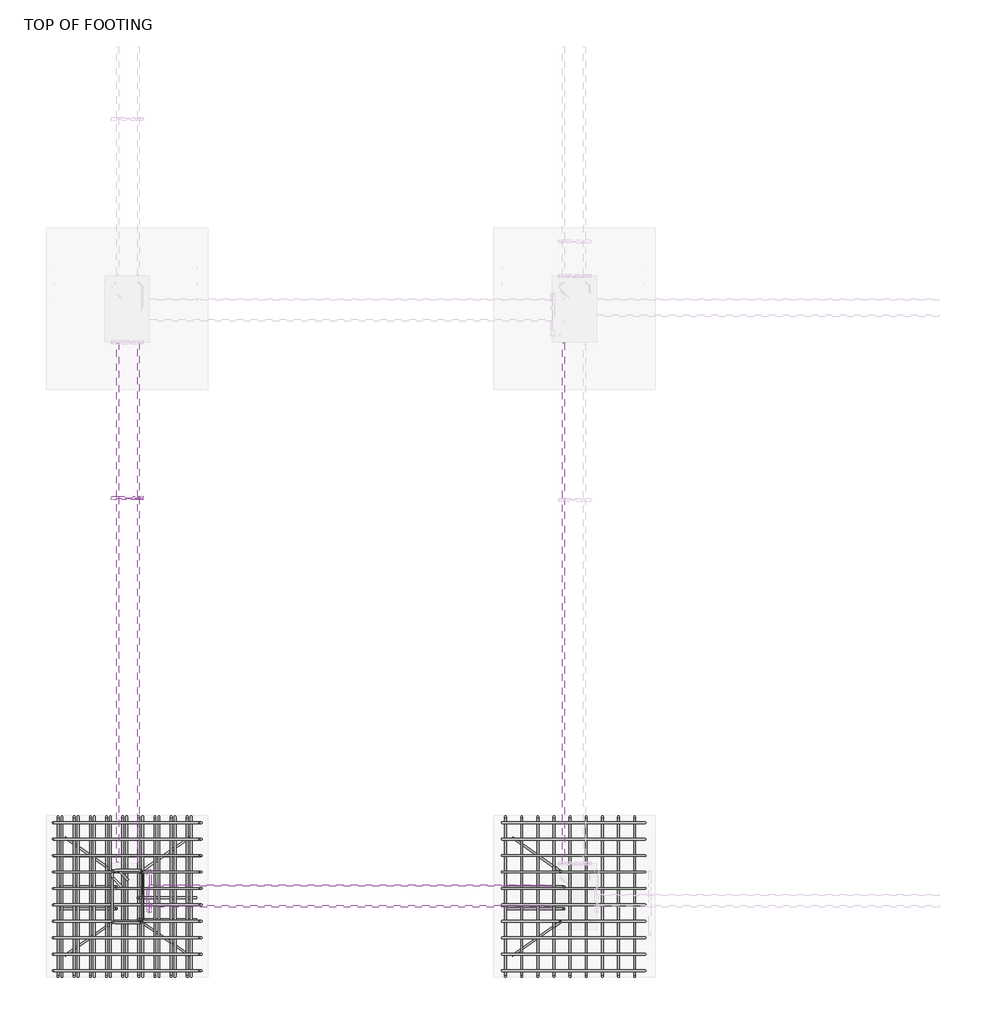
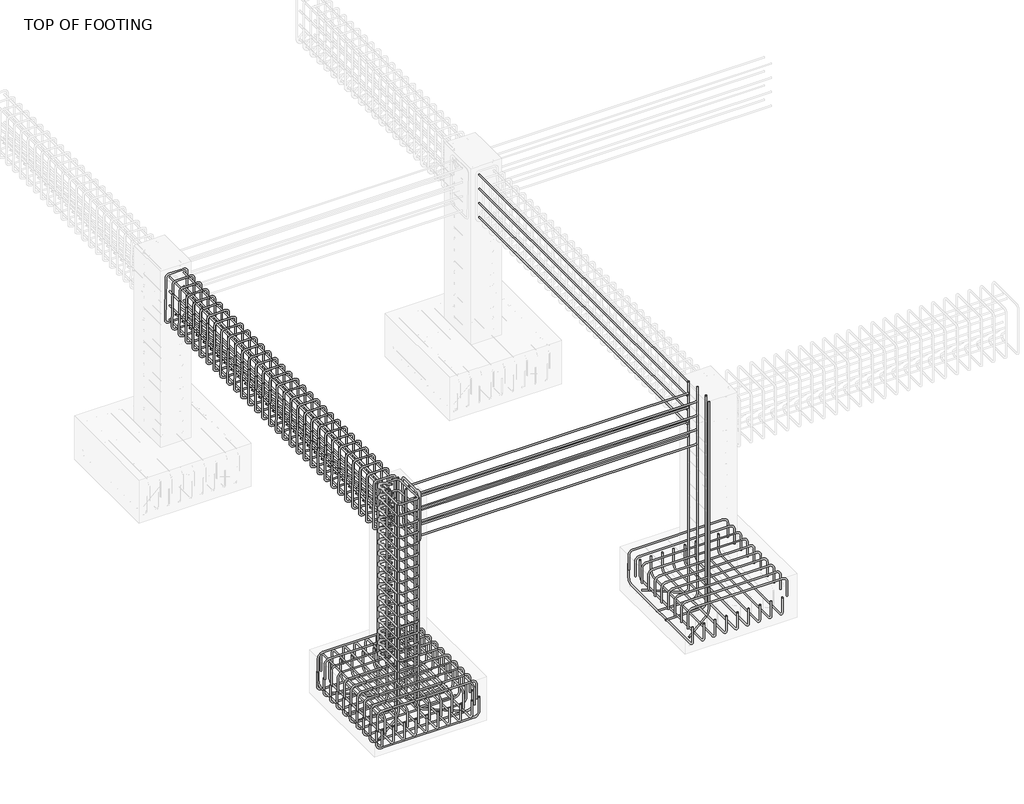
# One storey, part 2 of 18: 23 reinforcing bars.
"""IFC4 building model written with IfcOpenShell, lengths in millimetres."""

from ifc_helpers import new_model, si_unit, point, frame, origin, place, context, project, spatial, polyline, circle_curve, trimmed, segment, composite_curve, source, transform, mapped, element, save
from ifc_brep_helpers import swept_disk

model = new_model("IFC4")

# Units and contexts
model_context = context("Model", 3, world=origin())
ifc_project = project(units=[si_unit("LENGTHUNIT", "METRE", prefix="MILLI")], contexts=[model_context])

# Site, building, storey
site = spatial("IfcSite", under=ifc_project)
building = spatial("IfcBuilding", under=site)
storey = spatial("IfcBuildingStorey", under=building, Name="TOP OF FOOTING", Elevation=-1828.8)

# Reinforcing bars
placement = place(None, origin())
reinforcing_bar_shape = source(origin(), model_context, "Body", "SolidModel", [
    swept_disk(composite_curve([segment(polyline([(-11115.9859643, 5574.8477614, -40.0), (-11115.9859643, 5574.8477614, -2185.2530621)]), True, "CONTINUOUS"), segment(trimmed(circle_curve(frame((-11162.3359643, 5574.8477614, -2185.2530621), z_axis=(0.0, 1.0, 0.0), x_axis=(46.350000000000364, 0.0, 0.0)), 46.35), [point((-11115.9859643, 5574.8477614, -2185.2530621))], [point((-11162.3359643, 5574.8477614, -2231.6030621))], True, "CARTESIAN"), True, "CONTINUOUS"), segment(polyline([(-11162.3359643, 5574.8477614, -2231.6030621), (-11513.5126143, 5574.8477614, -2231.6030621)]), True, "CONTINUOUS")], self_intersect=False), 6.35),
])
element("IfcReinforcingBar", 1, at=placement, inside=storey, context=model_context, shape_type="MappedRepresentation", body=[
    mapped(reinforcing_bar_shape, transform((0.0, 0.0, 0.0), x_axis=(1.0, 0.0, 0.0), y_axis=(0.0, 1.0, 0.0), z_axis=(0.0, 0.0, 1.0))),
    mapped(reinforcing_bar_shape, transform((0.0, 148.3194112, 0.0), x_axis=(1.0, 0.0, 0.0), y_axis=(0.0, 1.0, 0.0), z_axis=(0.0, 0.0, 1.0))),
])
element("IfcReinforcingBar", 2, at=placement, inside=storey, context=model_context, shape_type="SolidModel", body=[
    swept_disk(composite_curve([segment(polyline([(-11140.9859643, 5830.3098681, -40.0), (-11140.9859643, 5830.3098681, -2185.2530621)]), True, "CONTINUOUS"), segment(trimmed(circle_curve(frame((-11178.9536616, 5856.895136, -2185.2530621), z_axis=(0.5735764363510553, 0.8191520442889855, 0.0), x_axis=(37.96769730000051, -26.585267899999963, 0.0)), 46.35), [point((-11140.9859643, 5830.3098681, -2185.2530621))], [point((-11178.9536616, 5856.895136, -2231.6030621))], True, "CARTESIAN"), True, "CONTINUOUS"), segment(polyline([(-11178.9536616, 5856.895136, -2231.6030621), (-11466.6207323, 6058.3217874, -2231.6030621)]), True, "CONTINUOUS")], self_intersect=False), 6.35),
])
reinforcing_bar_2_shape = source(origin(), model_context, "Body", "SolidModel", [
    swept_disk(composite_curve([segment(polyline([(-11036.6954038, 5770.3841028, -1782.45), (-11092.4389667, 5826.1276657, -1782.45)]), True, "CONTINUOUS"), segment(trimmed(circle_curve(frame((-11114.6067643, 5803.9598681, -1782.45), z_axis=(0.0, 0.0, 1.0), x_axis=(22.167797600000995, 22.167797600000085, 0.0)), 31.35), [point((-11092.4389667, 5826.1276657, -1782.45))], [point((-11145.9567643, 5803.9598681, -1782.45))], True, "CARTESIAN"), True, "CONTINUOUS"), segment(polyline([(-11145.9567643, 5803.9598681, -1782.45), (-11145.9567643, 5509.3598681, -1782.45)]), True, "CONTINUOUS"), segment(trimmed(circle_curve(frame((-11114.6067643, 5509.3598681, -1782.45), z_axis=(0.0, 0.0, 1.0), x_axis=(-31.349999999998545, 0.0, 0.0)), 31.35), [point((-11145.9567643, 5509.3598681, -1782.45))], [point((-11114.6067643, 5478.0098681, -1782.45))], True, "CARTESIAN"), True, "CONTINUOUS"), segment(polyline([(-11114.6067643, 5478.0098681, -1782.45), (-10970.0067643, 5478.0098681, -1782.45)]), True, "CONTINUOUS"), segment(trimmed(circle_curve(frame((-10970.0067643, 5509.3400831, -1783.5636125), z_axis=(0.0, 0.03552192833448201, 0.9993688971583016), x_axis=(0.0, -31.330214999999953, 1.1136125000000447)), 31.35), [point((-10970.0067643, 5478.0098681, -1782.45))], [point((-10938.6567643, 5509.3400831, -1783.5636125))], True, "CARTESIAN"), True, "CONTINUOUS"), segment(polyline([(-10938.6567643, 5509.3400831, -1783.5636125), (-10938.6567643, 5803.9796532, -1794.0363875)]), True, "CONTINUOUS"), segment(trimmed(circle_curve(frame((-10970.0067643, 5803.9796532, -1794.0363875), z_axis=(0.0, 0.03552192833448201, 0.9993688971583016), x_axis=(31.350000000000364, 0.0, 0.0)), 31.35), [point((-10938.6567643, 5803.9796532, -1794.0363875))], [point((-10970.0067643, 5835.3098681, -1795.15))], True, "CARTESIAN"), True, "CONTINUOUS"), segment(polyline([(-10970.0067643, 5835.3098681, -1795.15), (-11114.6067643, 5835.3098681, -1795.15)]), True, "CONTINUOUS"), segment(trimmed(circle_curve(frame((-11114.6067643, 5803.9598681, -1795.15), z_axis=(0.0, 0.0, 1.0), x_axis=(0.0, 31.350000000000364, 0.0)), 31.35), [point((-11114.6067643, 5835.3098681, -1795.15))], [point((-11136.7745619, 5781.7920705, -1795.15))], True, "CARTESIAN"), True, "CONTINUOUS"), segment(polyline([(-11136.7745619, 5781.7920705, -1795.15), (-11081.030999, 5726.0485076, -1795.15)]), True, "CONTINUOUS")], self_intersect=False), 6.35),
])
element("IfcReinforcingBar", 3, at=placement, inside=storey, context=model_context, shape_type="MappedRepresentation", body=[
    mapped(reinforcing_bar_2_shape, transform((0.0, 0.0, 0.0), x_axis=(1.0, 0.0, 0.0), y_axis=(0.0, 1.0, 0.0), z_axis=(0.0, 0.0, 1.0))),
    mapped(reinforcing_bar_2_shape, transform((0.0, 0.0, 116.0092918), x_axis=(1.0, 0.0, 0.0), y_axis=(0.0, 1.0, 0.0), z_axis=(0.0, 0.0, 1.0))),
    mapped(reinforcing_bar_2_shape, transform((0.0, 0.0, 232.0185836), x_axis=(1.0, 0.0, 0.0), y_axis=(0.0, 1.0, 0.0), z_axis=(0.0, 0.0, 1.0))),
    mapped(reinforcing_bar_2_shape, transform((0.0, 0.0, 348.0278755), x_axis=(1.0, 0.0, 0.0), y_axis=(0.0, 1.0, 0.0), z_axis=(0.0, 0.0, 1.0))),
    mapped(reinforcing_bar_2_shape, transform((0.0, 0.0, 464.0371673), x_axis=(1.0, 0.0, 0.0), y_axis=(0.0, 1.0, 0.0), z_axis=(0.0, 0.0, 1.0))),
    mapped(reinforcing_bar_2_shape, transform((0.0, 0.0, 580.0464591), x_axis=(1.0, 0.0, 0.0), y_axis=(0.0, 1.0, 0.0), z_axis=(0.0, 0.0, 1.0))),
    mapped(reinforcing_bar_2_shape, transform((0.0, 0.0, 696.0557509), x_axis=(1.0, 0.0, 0.0), y_axis=(0.0, 1.0, 0.0), z_axis=(0.0, 0.0, 1.0))),
    mapped(reinforcing_bar_2_shape, transform((0.0, 0.0, 812.0650428), x_axis=(1.0, 0.0, 0.0), y_axis=(0.0, 1.0, 0.0), z_axis=(0.0, 0.0, 1.0))),
    mapped(reinforcing_bar_2_shape, transform((0.0, 0.0, 928.0743346), x_axis=(1.0, 0.0, 0.0), y_axis=(0.0, 1.0, 0.0), z_axis=(0.0, 0.0, 1.0))),
    mapped(reinforcing_bar_2_shape, transform((0.0, 0.0, 1044.0836264), x_axis=(1.0, 0.0, 0.0), y_axis=(0.0, 1.0, 0.0), z_axis=(0.0, 0.0, 1.0))),
    mapped(reinforcing_bar_2_shape, transform((0.0, 0.0, 1160.0929182), x_axis=(1.0, 0.0, 0.0), y_axis=(0.0, 1.0, 0.0), z_axis=(0.0, 0.0, 1.0))),
    mapped(reinforcing_bar_2_shape, transform((0.0, 0.0, 1276.1022101), x_axis=(1.0, 0.0, 0.0), y_axis=(0.0, 1.0, 0.0), z_axis=(0.0, 0.0, 1.0))),
    mapped(reinforcing_bar_2_shape, transform((0.0, 0.0, 1392.1115019), x_axis=(1.0, 0.0, 0.0), y_axis=(0.0, 1.0, 0.0), z_axis=(0.0, 0.0, 1.0))),
    mapped(reinforcing_bar_2_shape, transform((0.0, 0.0, 1508.1207937), x_axis=(1.0, 0.0, 0.0), y_axis=(0.0, 1.0, 0.0), z_axis=(0.0, 0.0, 1.0))),
    mapped(reinforcing_bar_2_shape, transform((0.0, 0.0, 1624.1300855), x_axis=(1.0, 0.0, 0.0), y_axis=(0.0, 1.0, 0.0), z_axis=(0.0, 0.0, 1.0))),
    mapped(reinforcing_bar_2_shape, transform((0.0, 0.0, 1740.1393774), x_axis=(1.0, 0.0, 0.0), y_axis=(0.0, 1.0, 0.0), z_axis=(0.0, 0.0, 1.0))),
])
element("IfcReinforcingBar", 4, at=placement, inside=storey, context=model_context, shape_type="SolidModel", body=[
    swept_disk(composite_curve([segment(polyline([(-10943.6275643, 5830.3098681, -40.0), (-10943.6275643, 5830.3098681, -2185.2530621)]), True, "CONTINUOUS"), segment(trimmed(circle_curve(frame((-10905.6598671, 5856.895136, -2185.2530621), z_axis=(0.5735764363510552, -0.8191520442889856, 0.0), x_axis=(-37.96769720000157, -26.585267899999963, 0.0)), 46.35), [point((-10943.6275643, 5830.3098681, -2185.2530621))], [point((-10905.6598671, 5856.895136, -2231.6030621))], True, "CARTESIAN"), True, "CONTINUOUS"), segment(polyline([(-10905.6598671, 5856.895136, -2231.6030621), (-10617.9927964, 6058.3217874, -2231.6030621)]), True, "CONTINUOUS")], self_intersect=False), 6.35),
])
element("IfcReinforcingBar", 5, at=placement, inside=storey, context=model_context, shape_type="SolidModel", body=[
    swept_disk(composite_curve([segment(polyline([(-11140.9859643, 5483.0098681, -40.0), (-11140.9859643, 5483.0098681, -2185.2530621)]), True, "CONTINUOUS"), segment(trimmed(circle_curve(frame((-11178.9536616, 5456.4246003, -2185.2530621), z_axis=(-0.5735764363510105, 0.8191520442890168, 0.0), x_axis=(37.96769730000051, 26.58526780000011, 0.0)), 46.35), [point((-11140.9859643, 5483.0098681, -2185.2530621))], [point((-11178.9536616, 5456.4246003, -2231.6030621))], True, "CARTESIAN"), True, "CONTINUOUS"), segment(polyline([(-11178.9536616, 5456.4246003, -2231.6030621), (-11466.6207323, 5254.9979489, -2231.6030621)]), True, "CONTINUOUS")], self_intersect=False), 6.35),
])
element("IfcReinforcingBar", 6, at=placement, inside=storey, context=model_context, shape_type="SolidModel", body=[
    swept_disk(composite_curve([segment(polyline([(-10943.6275643, 5483.0098681, -40.0), (-10943.6275643, 5483.0098681, -2185.2530621)]), True, "CONTINUOUS"), segment(trimmed(circle_curve(frame((-10905.6598671, 5456.4246003, -2185.2530621), z_axis=(-0.5735764363510997, -0.8191520442889544, 0.0), x_axis=(-37.96769720000157, 26.58526780000011, 0.0)), 46.35), [point((-10943.6275643, 5483.0098681, -2185.2530621))], [point((-10905.6598671, 5456.4246003, -2231.6030621))], True, "CARTESIAN"), True, "CONTINUOUS"), segment(polyline([(-10905.6598671, 5456.4246003, -2231.6030621), (-10617.9927964, 5254.9979489, -2231.6030621)]), True, "CONTINUOUS")], self_intersect=False), 6.35),
])
reinforcing_bar_3_shape = source(origin(), model_context, "Body", "SolidModel", [
    swept_disk(composite_curve([segment(polyline([(-10968.6275643, 5499.8477614, -40.0), (-10968.6275643, 5499.8477614, -2185.2530621)]), True, "CONTINUOUS"), segment(trimmed(circle_curve(frame((-10922.2775643, 5499.8477614, -2185.2530621), z_axis=(0.0, -1.0, 0.0), x_axis=(-46.350000000000364, 0.0, 0.0)), 46.35), [point((-10968.6275643, 5499.8477614, -2185.2530621))], [point((-10922.2775643, 5499.8477614, -2231.6030621))], True, "CARTESIAN"), True, "CONTINUOUS"), segment(polyline([(-10922.2775643, 5499.8477614, -2231.6030621), (-10571.1009144, 5499.8477614, -2231.6030621)]), True, "CONTINUOUS")], self_intersect=False), 6.35),
])
element("IfcReinforcingBar", 7, at=placement, inside=storey, context=model_context, shape_type="MappedRepresentation", body=[
    mapped(reinforcing_bar_3_shape, transform((0.0, 0.0, 0.0), x_axis=(1.0, 0.0, 0.0), y_axis=(0.0, 1.0, 0.0), z_axis=(0.0, 0.0, 1.0))),
    mapped(reinforcing_bar_3_shape, transform((0.0, 148.3194112, 0.0), x_axis=(1.0, 0.0, 0.0), y_axis=(0.0, 1.0, 0.0), z_axis=(0.0, 0.0, 1.0))),
])
reinforcing_bar_4_shape = source(origin(), model_context, "Body", "SolidModel", [
    swept_disk(composite_curve([segment(polyline([(-8067.9859643, 5574.8477614, -40.0), (-8067.9859643, 5574.8477614, -2185.2530621)]), True, "CONTINUOUS"), segment(trimmed(circle_curve(frame((-8114.3359643, 5574.8477614, -2185.2530621), z_axis=(0.0, 1.0, 0.0), x_axis=(46.350000000000364, 0.0, 0.0)), 46.35), [point((-8067.9859643, 5574.8477614, -2185.2530621))], [point((-8114.3359643, 5574.8477614, -2231.6030621))], True, "CARTESIAN"), True, "CONTINUOUS"), segment(polyline([(-8114.3359643, 5574.8477614, -2231.6030621), (-8465.5126143, 5574.8477614, -2231.6030621)]), True, "CONTINUOUS")], self_intersect=False), 6.35),
])
element("IfcReinforcingBar", 8, at=placement, inside=storey, context=model_context, shape_type="MappedRepresentation", body=[
    mapped(reinforcing_bar_4_shape, transform((0.0, 0.0, 0.0), x_axis=(1.0, 0.0, 0.0), y_axis=(0.0, 1.0, 0.0), z_axis=(0.0, 0.0, 1.0))),
    mapped(reinforcing_bar_4_shape, transform((0.0, 148.3194112, 0.0), x_axis=(1.0, 0.0, 0.0), y_axis=(0.0, 1.0, 0.0), z_axis=(0.0, 0.0, 1.0))),
])
element("IfcReinforcingBar", 9, at=placement, inside=storey, context=model_context, shape_type="SolidModel", body=[
    swept_disk(composite_curve([segment(polyline([(-8092.9859643, 5830.3098681, -40.0), (-8092.9859643, 5830.3098681, -2185.2530621)]), True, "CONTINUOUS"), segment(trimmed(circle_curve(frame((-8130.9536616, 5856.895136, -2185.2530621), z_axis=(0.5735764363510552, 0.8191520442889856, 0.0), x_axis=(37.9676972999996, -26.585267899999963, 0.0)), 46.35), [point((-8092.9859643, 5830.3098681, -2185.2530621))], [point((-8130.9536616, 5856.895136, -2231.6030621))], True, "CARTESIAN"), True, "CONTINUOUS"), segment(polyline([(-8130.9536616, 5856.895136, -2231.6030621), (-8418.6207323, 6058.3217874, -2231.6030621)]), True, "CONTINUOUS")], self_intersect=False), 6.35),
])
element("IfcReinforcingBar", 10, at=placement, inside=storey, context=model_context, shape_type="SolidModel", body=[
    swept_disk(composite_curve([segment(polyline([(-8092.9859643, 5483.0098681, -40.0), (-8092.9859643, 5483.0098681, -2185.2530621)]), True, "CONTINUOUS"), segment(trimmed(circle_curve(frame((-8130.9536616, 5456.4246003, -2185.2530621), z_axis=(-0.5735764363510105, 0.8191520442890168, 0.0), x_axis=(37.9676972999996, 26.58526780000011, 0.0)), 46.35), [point((-8092.9859643, 5483.0098681, -2185.2530621))], [point((-8130.9536616, 5456.4246003, -2231.6030621))], True, "CARTESIAN"), True, "CONTINUOUS"), segment(polyline([(-8130.9536616, 5456.4246003, -2231.6030621), (-8418.6207323, 5254.9979489, -2231.6030621)]), True, "CONTINUOUS")], self_intersect=False), 6.35),
])
reinforcing_bar_5_shape = source(origin(), model_context, "Body", "SolidModel", [
    swept_disk(composite_curve([segment(polyline([(-8488.4399078, 6160.3098681, -2056.7800629), (-8488.4399078, 6160.3098681, -1909.4800629)]), True, "CONTINUOUS"), segment(trimmed(circle_curve(frame((-8442.0899078, 6160.3098681, -1909.4800629), z_axis=(0.0, 1.0, 0.0), x_axis=(-46.350000000000364, 0.0, 0.0)), 46.35), [point((-8488.4399078, 6160.3098681, -1909.4800629))], [point((-8442.0899078, 6160.3098681, -1863.1300629))], True, "CARTESIAN"), True, "CONTINUOUS"), segment(polyline([(-8442.0899078, 6160.3098681, -1863.1300629), (-7562.3320898, 6160.3098681, -1863.1300629)]), True, "CONTINUOUS"), segment(trimmed(circle_curve(frame((-7562.3320898, 6160.3098681, -1909.4800629), z_axis=(0.0, 1.0, 0.0), x_axis=(0.0, 0.0, 46.34999999999991)), 46.35), [point((-7562.3320898, 6160.3098681, -1863.1300629))], [point((-7515.9820898, 6160.3098681, -1909.4800629))], True, "CARTESIAN"), True, "CONTINUOUS"), segment(polyline([(-7515.9820898, 6160.3098681, -1909.4800629), (-7515.9820898, 6160.3098681, -2056.7800629)]), True, "CONTINUOUS")], self_intersect=False), 6.35),
])
element("IfcReinforcingBar", 11, at=placement, inside=storey, context=model_context, shape_type="MappedRepresentation", body=[
    mapped(reinforcing_bar_5_shape, transform((0.0, 0.0, 0.0), x_axis=(1.0, 0.0, 0.0), y_axis=(0.0, 1.0, 0.0), z_axis=(0.0, 0.0, 1.0))),
    mapped(reinforcing_bar_5_shape, transform((0.0, -111.9222222, 0.0), x_axis=(1.0, 0.0, 0.0), y_axis=(0.0, 1.0, 0.0), z_axis=(0.0, 0.0, 1.0))),
    mapped(reinforcing_bar_5_shape, transform((0.0, -223.8444444, 0.0), x_axis=(1.0, 0.0, 0.0), y_axis=(0.0, 1.0, 0.0), z_axis=(0.0, 0.0, 1.0))),
    mapped(reinforcing_bar_5_shape, transform((0.0, -335.7666667, 0.0), x_axis=(1.0, 0.0, 0.0), y_axis=(0.0, 1.0, 0.0), z_axis=(0.0, 0.0, 1.0))),
    mapped(reinforcing_bar_5_shape, transform((0.0, -447.6888889, 0.0), x_axis=(1.0, 0.0, 0.0), y_axis=(0.0, 1.0, 0.0), z_axis=(0.0, 0.0, 1.0))),
    mapped(reinforcing_bar_5_shape, transform((0.0, -559.6111111, 0.0), x_axis=(1.0, 0.0, 0.0), y_axis=(0.0, 1.0, 0.0), z_axis=(0.0, 0.0, 1.0))),
    mapped(reinforcing_bar_5_shape, transform((0.0, -671.5333333, 0.0), x_axis=(1.0, 0.0, 0.0), y_axis=(0.0, 1.0, 0.0), z_axis=(0.0, 0.0, 1.0))),
    mapped(reinforcing_bar_5_shape, transform((0.0, -783.4555556, 0.0), x_axis=(1.0, 0.0, 0.0), y_axis=(0.0, 1.0, 0.0), z_axis=(0.0, 0.0, 1.0))),
    mapped(reinforcing_bar_5_shape, transform((0.0, -895.3777778, 0.0), x_axis=(1.0, 0.0, 0.0), y_axis=(0.0, 1.0, 0.0), z_axis=(0.0, 0.0, 1.0))),
    mapped(reinforcing_bar_5_shape, transform((0.0, -1007.3, 0.0), x_axis=(1.0, 0.0, 0.0), y_axis=(0.0, 1.0, 0.0), z_axis=(0.0, 0.0, 1.0))),
])
reinforcing_bar_6_shape = source(origin(), model_context, "Body", "SolidModel", [
    swept_disk(composite_curve([segment(polyline([(-8465.5126143, 6200.3098681, -2025.2530621), (-8465.5126143, 6200.3098681, -2172.5530621)]), True, "CONTINUOUS"), segment(trimmed(circle_curve(frame((-8465.5126143, 6153.9598681, -2172.5530621), z_axis=(-1.0, 0.0, 0.0), x_axis=(0.0, 46.350000000000364, 0.0)), 46.35), [point((-8465.5126143, 6200.3098681, -2172.5530621))], [point((-8465.5126143, 6153.9598681, -2218.9030621))], True, "CARTESIAN"), True, "CONTINUOUS"), segment(polyline([(-8465.5126143, 6153.9598681, -2218.9030621), (-8465.5126143, 5159.3598681, -2218.9030621)]), True, "CONTINUOUS"), segment(trimmed(circle_curve(frame((-8465.5126143, 5159.3598681, -2172.5530621), z_axis=(-1.0, 0.0, 0.0), x_axis=(0.0, 0.0, -46.350000000000364)), 46.35), [point((-8465.5126143, 5159.3598681, -2218.9030621))], [point((-8465.5126143, 5113.0098681, -2172.5530621))], True, "CARTESIAN"), True, "CONTINUOUS"), segment(polyline([(-8465.5126143, 5113.0098681, -2172.5530621), (-8465.5126143, 5113.0098681, -2025.2530621)]), True, "CONTINUOUS")], self_intersect=False), 6.35),
])
element("IfcReinforcingBar", 12, at=placement, inside=storey, context=model_context, shape_type="MappedRepresentation", body=[
    mapped(reinforcing_bar_6_shape, transform((0.0, 0.0, 0.0), x_axis=(1.0, 0.0, 0.0), y_axis=(0.0, 1.0, 0.0), z_axis=(0.0, 0.0, 1.0))),
    mapped(reinforcing_bar_6_shape, transform((109.9890349, 0.0, 0.0), x_axis=(1.0, 0.0, 0.0), y_axis=(0.0, 1.0, 0.0), z_axis=(0.0, 0.0, 1.0))),
    mapped(reinforcing_bar_6_shape, transform((219.9780699, 0.0, 0.0), x_axis=(1.0, 0.0, 0.0), y_axis=(0.0, 1.0, 0.0), z_axis=(0.0, 0.0, 1.0))),
    mapped(reinforcing_bar_6_shape, transform((329.9671048, 0.0, 0.0), x_axis=(1.0, 0.0, 0.0), y_axis=(0.0, 1.0, 0.0), z_axis=(0.0, 0.0, 1.0))),
    mapped(reinforcing_bar_6_shape, transform((439.9561397, 0.0, 0.0), x_axis=(1.0, 0.0, 0.0), y_axis=(0.0, 1.0, 0.0), z_axis=(0.0, 0.0, 1.0))),
    mapped(reinforcing_bar_6_shape, transform((549.9451746, 0.0, 0.0), x_axis=(1.0, 0.0, 0.0), y_axis=(0.0, 1.0, 0.0), z_axis=(0.0, 0.0, 1.0))),
    mapped(reinforcing_bar_6_shape, transform((659.9342096, 0.0, 0.0), x_axis=(1.0, 0.0, 0.0), y_axis=(0.0, 1.0, 0.0), z_axis=(0.0, 0.0, 1.0))),
    mapped(reinforcing_bar_6_shape, transform((769.9232445, 0.0, 0.0), x_axis=(1.0, 0.0, 0.0), y_axis=(0.0, 1.0, 0.0), z_axis=(0.0, 0.0, 1.0))),
    mapped(reinforcing_bar_6_shape, transform((879.9122794, 0.0, 0.0), x_axis=(1.0, 0.0, 0.0), y_axis=(0.0, 1.0, 0.0), z_axis=(0.0, 0.0, 1.0))),
])
reinforcing_bar_7_shape = source(origin(), model_context, "Body", "SolidModel", [
    swept_disk(composite_curve([segment(polyline([(-10538.6567643, 6160.3098681, -2046.8654906), (-10538.6567643, 6160.3098681, -2194.1654906)]), True, "CONTINUOUS"), segment(trimmed(circle_curve(frame((-10585.0067643, 6160.3098681, -2194.1654906), z_axis=(0.0, 1.0, 0.0), x_axis=(46.350000000000364, 0.0, 0.0)), 46.35), [point((-10538.6567643, 6160.3098681, -2194.1654906))], [point((-10585.0067643, 6160.3098681, -2240.5154906))], True, "CARTESIAN"), True, "CONTINUOUS"), segment(polyline([(-10585.0067643, 6160.3098681, -2240.5154906), (-11499.6067643, 6160.3098681, -2240.5154906)]), True, "CONTINUOUS"), segment(trimmed(circle_curve(frame((-11499.6067643, 6160.3098681, -2194.1654906), z_axis=(0.0, 1.0, 0.0), x_axis=(0.0, 0.0, -46.34999999999991)), 46.35), [point((-11499.6067643, 6160.3098681, -2240.5154906))], [point((-11545.9567643, 6160.3098681, -2194.1654906))], True, "CARTESIAN"), True, "CONTINUOUS"), segment(polyline([(-11545.9567643, 6160.3098681, -2194.1654906), (-11545.9567643, 6160.3098681, -2046.8654906)]), True, "CONTINUOUS")], self_intersect=False), 6.35),
])
element("IfcReinforcingBar", 13, at=placement, inside=storey, context=model_context, shape_type="MappedRepresentation", body=[
    mapped(reinforcing_bar_7_shape, transform((0.0, 0.0, 0.0), x_axis=(1.0, 0.0, 0.0), y_axis=(0.0, 1.0, 0.0), z_axis=(0.0, 0.0, 1.0))),
    mapped(reinforcing_bar_7_shape, transform((0.0, -111.9222222, 0.0), x_axis=(1.0, 0.0, 0.0), y_axis=(0.0, 1.0, 0.0), z_axis=(0.0, 0.0, 1.0))),
    mapped(reinforcing_bar_7_shape, transform((0.0, -223.8444444, 0.0), x_axis=(1.0, 0.0, 0.0), y_axis=(0.0, 1.0, 0.0), z_axis=(0.0, 0.0, 1.0))),
    mapped(reinforcing_bar_7_shape, transform((0.0, -335.7666667, 0.0), x_axis=(1.0, 0.0, 0.0), y_axis=(0.0, 1.0, 0.0), z_axis=(0.0, 0.0, 1.0))),
    mapped(reinforcing_bar_7_shape, transform((0.0, -447.6888889, 0.0), x_axis=(1.0, 0.0, 0.0), y_axis=(0.0, 1.0, 0.0), z_axis=(0.0, 0.0, 1.0))),
    mapped(reinforcing_bar_7_shape, transform((0.0, -559.6111111, 0.0), x_axis=(1.0, 0.0, 0.0), y_axis=(0.0, 1.0, 0.0), z_axis=(0.0, 0.0, 1.0))),
    mapped(reinforcing_bar_7_shape, transform((0.0, -671.5333333, 0.0), x_axis=(1.0, 0.0, 0.0), y_axis=(0.0, 1.0, 0.0), z_axis=(0.0, 0.0, 1.0))),
    mapped(reinforcing_bar_7_shape, transform((0.0, -783.4555556, 0.0), x_axis=(1.0, 0.0, 0.0), y_axis=(0.0, 1.0, 0.0), z_axis=(0.0, 0.0, 1.0))),
    mapped(reinforcing_bar_7_shape, transform((0.0, -895.3777778, 0.0), x_axis=(1.0, 0.0, 0.0), y_axis=(0.0, 1.0, 0.0), z_axis=(0.0, 0.0, 1.0))),
    mapped(reinforcing_bar_7_shape, transform((0.0, -1007.3, 0.0), x_axis=(1.0, 0.0, 0.0), y_axis=(0.0, 1.0, 0.0), z_axis=(0.0, 0.0, 1.0))),
])
reinforcing_bar_8_shape = source(origin(), model_context, "Body", "SolidModel", [
    swept_disk(composite_curve([segment(polyline([(-11536.4399078, 6160.3098681, -2056.7800629), (-11536.4399078, 6160.3098681, -1909.4800629)]), True, "CONTINUOUS"), segment(trimmed(circle_curve(frame((-11490.0899078, 6160.3098681, -1909.4800629), z_axis=(0.0, 1.0, 0.0), x_axis=(-46.350000000000364, 0.0, 0.0)), 46.35), [point((-11536.4399078, 6160.3098681, -1909.4800629))], [point((-11490.0899078, 6160.3098681, -1863.1300629))], True, "CARTESIAN"), True, "CONTINUOUS"), segment(polyline([(-11490.0899078, 6160.3098681, -1863.1300629), (-10610.3320898, 6160.3098681, -1863.1300629)]), True, "CONTINUOUS"), segment(trimmed(circle_curve(frame((-10610.3320898, 6160.3098681, -1909.4800629), z_axis=(0.0, 1.0, 0.0), x_axis=(0.0, 0.0, 46.34999999999991)), 46.35), [point((-10610.3320898, 6160.3098681, -1863.1300629))], [point((-10563.9820898, 6160.3098681, -1909.4800629))], True, "CARTESIAN"), True, "CONTINUOUS"), segment(polyline([(-10563.9820898, 6160.3098681, -1909.4800629), (-10563.9820898, 6160.3098681, -2056.7800629)]), True, "CONTINUOUS")], self_intersect=False), 6.35),
])
element("IfcReinforcingBar", 14, at=placement, inside=storey, context=model_context, shape_type="MappedRepresentation", body=[
    mapped(reinforcing_bar_8_shape, transform((0.0, 0.0, 0.0), x_axis=(1.0, 0.0, 0.0), y_axis=(0.0, 1.0, 0.0), z_axis=(0.0, 0.0, 1.0))),
    mapped(reinforcing_bar_8_shape, transform((0.0, -111.9222222, 0.0), x_axis=(1.0, 0.0, 0.0), y_axis=(0.0, 1.0, 0.0), z_axis=(0.0, 0.0, 1.0))),
    mapped(reinforcing_bar_8_shape, transform((0.0, -223.8444444, 0.0), x_axis=(1.0, 0.0, 0.0), y_axis=(0.0, 1.0, 0.0), z_axis=(0.0, 0.0, 1.0))),
    mapped(reinforcing_bar_8_shape, transform((0.0, -335.7666667, 0.0), x_axis=(1.0, 0.0, 0.0), y_axis=(0.0, 1.0, 0.0), z_axis=(0.0, 0.0, 1.0))),
    mapped(reinforcing_bar_8_shape, transform((0.0, -447.6888889, 0.0), x_axis=(1.0, 0.0, 0.0), y_axis=(0.0, 1.0, 0.0), z_axis=(0.0, 0.0, 1.0))),
    mapped(reinforcing_bar_8_shape, transform((0.0, -559.6111111, 0.0), x_axis=(1.0, 0.0, 0.0), y_axis=(0.0, 1.0, 0.0), z_axis=(0.0, 0.0, 1.0))),
    mapped(reinforcing_bar_8_shape, transform((0.0, -671.5333333, 0.0), x_axis=(1.0, 0.0, 0.0), y_axis=(0.0, 1.0, 0.0), z_axis=(0.0, 0.0, 1.0))),
    mapped(reinforcing_bar_8_shape, transform((0.0, -783.4555556, 0.0), x_axis=(1.0, 0.0, 0.0), y_axis=(0.0, 1.0, 0.0), z_axis=(0.0, 0.0, 1.0))),
    mapped(reinforcing_bar_8_shape, transform((0.0, -895.3777778, 0.0), x_axis=(1.0, 0.0, 0.0), y_axis=(0.0, 1.0, 0.0), z_axis=(0.0, 0.0, 1.0))),
    mapped(reinforcing_bar_8_shape, transform((0.0, -1007.3, 0.0), x_axis=(1.0, 0.0, 0.0), y_axis=(0.0, 1.0, 0.0), z_axis=(0.0, 0.0, 1.0))),
])
reinforcing_bar_9_shape = source(origin(), model_context, "Body", "SolidModel", [
    swept_disk(composite_curve([segment(polyline([(-10607.1065918, 6200.3098681, -2080.1793981), (-10607.1065918, 6200.3098681, -1932.8793981)]), True, "CONTINUOUS"), segment(trimmed(circle_curve(frame((-10607.1065918, 6153.9598681, -1932.8793981), z_axis=(1.0, 0.0, 0.0), x_axis=(0.0, 46.350000000000364, 0.0)), 46.35), [point((-10607.1065918, 6200.3098681, -1932.8793981))], [point((-10607.1065918, 6153.9598681, -1886.5293981))], True, "CARTESIAN"), True, "CONTINUOUS"), segment(polyline([(-10607.1065918, 6153.9598681, -1886.5293981), (-10607.1065918, 5159.3598681, -1886.5293981)]), True, "CONTINUOUS"), segment(trimmed(circle_curve(frame((-10607.1065918, 5159.3598681, -1932.8793981), z_axis=(1.0, 0.0, 0.0), x_axis=(0.0, 0.0, 46.34999999999991)), 46.35), [point((-10607.1065918, 5159.3598681, -1886.5293981))], [point((-10607.1065918, 5113.0098681, -1932.8793981))], True, "CARTESIAN"), True, "CONTINUOUS"), segment(polyline([(-10607.1065918, 5113.0098681, -1932.8793981), (-10607.1065918, 5113.0098681, -2080.1793981)]), True, "CONTINUOUS")], self_intersect=False), 6.35),
])
element("IfcReinforcingBar", 15, at=placement, inside=storey, context=model_context, shape_type="MappedRepresentation", body=[
    mapped(reinforcing_bar_9_shape, transform((0.0, 0.0, 0.0), x_axis=(1.0, 0.0, 0.0), y_axis=(0.0, 1.0, 0.0), z_axis=(0.0, 0.0, 1.0))),
    mapped(reinforcing_bar_9_shape, transform((-109.9785589, 0.0, 0.0), x_axis=(1.0, 0.0, 0.0), y_axis=(0.0, 1.0, 0.0), z_axis=(0.0, 0.0, 1.0))),
    mapped(reinforcing_bar_9_shape, transform((-219.9571177, 0.0, 0.0), x_axis=(1.0, 0.0, 0.0), y_axis=(0.0, 1.0, 0.0), z_axis=(0.0, 0.0, 1.0))),
    mapped(reinforcing_bar_9_shape, transform((-329.9356766, 0.0, 0.0), x_axis=(1.0, 0.0, 0.0), y_axis=(0.0, 1.0, 0.0), z_axis=(0.0, 0.0, 1.0))),
    mapped(reinforcing_bar_9_shape, transform((-439.9142355, 0.0, 0.0), x_axis=(1.0, 0.0, 0.0), y_axis=(0.0, 1.0, 0.0), z_axis=(0.0, 0.0, 1.0))),
    mapped(reinforcing_bar_9_shape, transform((-549.8927943, 0.0, 0.0), x_axis=(1.0, 0.0, 0.0), y_axis=(0.0, 1.0, 0.0), z_axis=(0.0, 0.0, 1.0))),
    mapped(reinforcing_bar_9_shape, transform((-659.8713532, 0.0, 0.0), x_axis=(1.0, 0.0, 0.0), y_axis=(0.0, 1.0, 0.0), z_axis=(0.0, 0.0, 1.0))),
    mapped(reinforcing_bar_9_shape, transform((-769.8499121, 0.0, 0.0), x_axis=(1.0, 0.0, 0.0), y_axis=(0.0, 1.0, 0.0), z_axis=(0.0, 0.0, 1.0))),
    mapped(reinforcing_bar_9_shape, transform((-879.828471, 0.0, 0.0), x_axis=(1.0, 0.0, 0.0), y_axis=(0.0, 1.0, 0.0), z_axis=(0.0, 0.0, 1.0))),
])
reinforcing_bar_10_shape = source(origin(), model_context, "Body", "SolidModel", [
    swept_disk(composite_curve([segment(polyline([(-11513.5126143, 6200.3098681, -2025.2530621), (-11513.5126143, 6200.3098681, -2172.5530621)]), True, "CONTINUOUS"), segment(trimmed(circle_curve(frame((-11513.5126143, 6153.9598681, -2172.5530621), z_axis=(-1.0, 0.0, 0.0), x_axis=(0.0, 46.350000000000364, 0.0)), 46.35), [point((-11513.5126143, 6200.3098681, -2172.5530621))], [point((-11513.5126143, 6153.9598681, -2218.9030621))], True, "CARTESIAN"), True, "CONTINUOUS"), segment(polyline([(-11513.5126143, 6153.9598681, -2218.9030621), (-11513.5126143, 5159.3598681, -2218.9030621)]), True, "CONTINUOUS"), segment(trimmed(circle_curve(frame((-11513.5126143, 5159.3598681, -2172.5530621), z_axis=(-1.0, 0.0, 0.0), x_axis=(0.0, 0.0, -46.350000000000364)), 46.35), [point((-11513.5126143, 5159.3598681, -2218.9030621))], [point((-11513.5126143, 5113.0098681, -2172.5530621))], True, "CARTESIAN"), True, "CONTINUOUS"), segment(polyline([(-11513.5126143, 5113.0098681, -2172.5530621), (-11513.5126143, 5113.0098681, -2025.2530621)]), True, "CONTINUOUS")], self_intersect=False), 6.35),
])
element("IfcReinforcingBar", 16, at=placement, inside=storey, context=model_context, shape_type="MappedRepresentation", body=[
    mapped(reinforcing_bar_10_shape, transform((0.0, 0.0, 0.0), x_axis=(1.0, 0.0, 0.0), y_axis=(0.0, 1.0, 0.0), z_axis=(0.0, 0.0, 1.0))),
    mapped(reinforcing_bar_10_shape, transform((109.9890349, 0.0, 0.0), x_axis=(1.0, 0.0, 0.0), y_axis=(0.0, 1.0, 0.0), z_axis=(0.0, 0.0, 1.0))),
    mapped(reinforcing_bar_10_shape, transform((219.9780699, 0.0, 0.0), x_axis=(1.0, 0.0, 0.0), y_axis=(0.0, 1.0, 0.0), z_axis=(0.0, 0.0, 1.0))),
    mapped(reinforcing_bar_10_shape, transform((329.9671048, 0.0, 0.0), x_axis=(1.0, 0.0, 0.0), y_axis=(0.0, 1.0, 0.0), z_axis=(0.0, 0.0, 1.0))),
    mapped(reinforcing_bar_10_shape, transform((439.9561397, 0.0, 0.0), x_axis=(1.0, 0.0, 0.0), y_axis=(0.0, 1.0, 0.0), z_axis=(0.0, 0.0, 1.0))),
    mapped(reinforcing_bar_10_shape, transform((549.9451746, 0.0, 0.0), x_axis=(1.0, 0.0, 0.0), y_axis=(0.0, 1.0, 0.0), z_axis=(0.0, 0.0, 1.0))),
    mapped(reinforcing_bar_10_shape, transform((659.9342096, 0.0, 0.0), x_axis=(1.0, 0.0, 0.0), y_axis=(0.0, 1.0, 0.0), z_axis=(0.0, 0.0, 1.0))),
    mapped(reinforcing_bar_10_shape, transform((769.9232445, 0.0, 0.0), x_axis=(1.0, 0.0, 0.0), y_axis=(0.0, 1.0, 0.0), z_axis=(0.0, 0.0, 1.0))),
    mapped(reinforcing_bar_10_shape, transform((879.9122794, 0.0, 0.0), x_axis=(1.0, 0.0, 0.0), y_axis=(0.0, 1.0, 0.0), z_axis=(0.0, 0.0, 1.0))),
])
reinforcing_bar_11_shape = source(origin(), model_context, "Body", "SolidModel", [
    swept_disk(composite_curve([segment(polyline([(-11047.9181249, 9425.3098681, -488.7242346), (-10992.1745619, 9425.3098681, -544.4677976)]), True, "CONTINUOUS"), segment(trimmed(circle_curve(frame((-10970.0067643, 9425.3098681, -522.3), z_axis=(0.0, -1.0, 0.0), x_axis=(-22.167797599999176, 0.0, -22.167797600000085)), 31.35), [point((-10992.1745619, 9425.3098681, -544.4677976))], [point((-10938.6567643, 9425.3098681, -522.3))], True, "CARTESIAN"), True, "CONTINUOUS"), segment(polyline([(-10938.6567643, 9425.3098681, -522.3), (-10938.6567643, 9425.3098681, -77.7)]), True, "CONTINUOUS"), segment(trimmed(circle_curve(frame((-10970.0067643, 9425.3098681, -77.7), z_axis=(0.0, -1.0, 0.0), x_axis=(31.350000000000364, 0.0, 0.0)), 31.35), [point((-10938.6567643, 9425.3098681, -77.7))], [point((-10970.0067643, 9425.3098681, -46.35))], True, "CARTESIAN"), True, "CONTINUOUS"), segment(polyline([(-10970.0067643, 9425.3098681, -46.35), (-11114.6067643, 9425.3098681, -46.35)]), True, "CONTINUOUS"), segment(trimmed(circle_curve(frame((-11114.6067643, 9426.0944538, -77.6901807), z_axis=(0.0, -0.9996867842138424, -0.025026655153786322), x_axis=(0.0, -0.7845857000011165, 31.340180699999998)), 31.35), [point((-11114.6067643, 9425.3098681, -46.35))], [point((-11145.9567643, 9426.0944538, -77.6901807))], True, "CARTESIAN"), True, "CONTINUOUS"), segment(polyline([(-11145.9567643, 9426.0944538, -77.6901807), (-11145.9567643, 9437.2252825, -522.3098193)]), True, "CONTINUOUS"), segment(trimmed(circle_curve(frame((-11114.6067643, 9437.2252825, -522.3098193), z_axis=(0.0, -0.9996867842138424, -0.025026655153786322), x_axis=(-31.349999999998545, 0.0, 0.0)), 31.35), [point((-11145.9567643, 9437.2252825, -522.3098193))], [point((-11114.6067643, 9438.0098681, -553.65))], True, "CARTESIAN"), True, "CONTINUOUS"), segment(polyline([(-11114.6067643, 9438.0098681, -553.65), (-10970.0067643, 9438.0098681, -553.65)]), True, "CONTINUOUS"), segment(trimmed(circle_curve(frame((-10970.0067643, 9438.0098681, -522.3), z_axis=(0.0, -1.0, 0.0), x_axis=(0.0, 0.0, -31.350000000000023)), 31.35), [point((-10970.0067643, 9438.0098681, -553.65))], [point((-10947.8389667, 9438.0098681, -500.1322024))], True, "CARTESIAN"), True, "CONTINUOUS"), segment(polyline([(-10947.8389667, 9438.0098681, -500.1322024), (-11003.5825297, 9438.0098681, -444.3886395)]), True, "CONTINUOUS")], self_intersect=False), 6.35),
])
element("IfcReinforcingBar", 17, at=placement, inside=storey, context=model_context, shape_type="MappedRepresentation", body=[
    mapped(reinforcing_bar_11_shape, transform((0.0, 0.0, 0.0), x_axis=(1.0, 0.0, 0.0), y_axis=(0.0, 1.0, 0.0), z_axis=(0.0, 0.0, 1.0))),
    mapped(reinforcing_bar_11_shape, transform((0.0, -117.91, 0.0), x_axis=(1.0, 0.0, 0.0), y_axis=(0.0, 1.0, 0.0), z_axis=(0.0, 0.0, 1.0))),
    mapped(reinforcing_bar_11_shape, transform((0.0, -235.82, 0.0), x_axis=(1.0, 0.0, 0.0), y_axis=(0.0, 1.0, 0.0), z_axis=(0.0, 0.0, 1.0))),
    mapped(reinforcing_bar_11_shape, transform((0.0, -353.7300001, 0.0), x_axis=(1.0, 0.0, 0.0), y_axis=(0.0, 1.0, 0.0), z_axis=(0.0, 0.0, 1.0))),
    mapped(reinforcing_bar_11_shape, transform((0.0, -471.6400001, 0.0), x_axis=(1.0, 0.0, 0.0), y_axis=(0.0, 1.0, 0.0), z_axis=(0.0, 0.0, 1.0))),
    mapped(reinforcing_bar_11_shape, transform((0.0, -589.5500001, 0.0), x_axis=(1.0, 0.0, 0.0), y_axis=(0.0, 1.0, 0.0), z_axis=(0.0, 0.0, 1.0))),
    mapped(reinforcing_bar_11_shape, transform((0.0, -707.4600001, 0.0), x_axis=(1.0, 0.0, 0.0), y_axis=(0.0, 1.0, 0.0), z_axis=(0.0, 0.0, 1.0))),
    mapped(reinforcing_bar_11_shape, transform((0.0, -825.3700001, 0.0), x_axis=(1.0, 0.0, 0.0), y_axis=(0.0, 1.0, 0.0), z_axis=(0.0, 0.0, 1.0))),
    mapped(reinforcing_bar_11_shape, transform((0.0, -943.2800002, 0.0), x_axis=(1.0, 0.0, 0.0), y_axis=(0.0, 1.0, 0.0), z_axis=(0.0, 0.0, 1.0))),
    mapped(reinforcing_bar_11_shape, transform((0.0, -1061.1900002, 0.0), x_axis=(1.0, 0.0, 0.0), y_axis=(0.0, 1.0, 0.0), z_axis=(0.0, 0.0, 1.0))),
    mapped(reinforcing_bar_11_shape, transform((0.0, -1179.1000002, 0.0), x_axis=(1.0, 0.0, 0.0), y_axis=(0.0, 1.0, 0.0), z_axis=(0.0, 0.0, 1.0))),
    mapped(reinforcing_bar_11_shape, transform((0.0, -1297.0100002, 0.0), x_axis=(1.0, 0.0, 0.0), y_axis=(0.0, 1.0, 0.0), z_axis=(0.0, 0.0, 1.0))),
    mapped(reinforcing_bar_11_shape, transform((0.0, -1414.9200002, 0.0), x_axis=(1.0, 0.0, 0.0), y_axis=(0.0, 1.0, 0.0), z_axis=(0.0, 0.0, 1.0))),
    mapped(reinforcing_bar_11_shape, transform((0.0, -1532.8300003, 0.0), x_axis=(1.0, 0.0, 0.0), y_axis=(0.0, 1.0, 0.0), z_axis=(0.0, 0.0, 1.0))),
    mapped(reinforcing_bar_11_shape, transform((0.0, -1650.7400003, 0.0), x_axis=(1.0, 0.0, 0.0), y_axis=(0.0, 1.0, 0.0), z_axis=(0.0, 0.0, 1.0))),
    mapped(reinforcing_bar_11_shape, transform((0.0, -1768.6500003, 0.0), x_axis=(1.0, 0.0, 0.0), y_axis=(0.0, 1.0, 0.0), z_axis=(0.0, 0.0, 1.0))),
    mapped(reinforcing_bar_11_shape, transform((0.0, -1886.5600003, 0.0), x_axis=(1.0, 0.0, 0.0), y_axis=(0.0, 1.0, 0.0), z_axis=(0.0, 0.0, 1.0))),
    mapped(reinforcing_bar_11_shape, transform((0.0, -2004.4700003, 0.0), x_axis=(1.0, 0.0, 0.0), y_axis=(0.0, 1.0, 0.0), z_axis=(0.0, 0.0, 1.0))),
    mapped(reinforcing_bar_11_shape, transform((0.0, -2122.3800004, 0.0), x_axis=(1.0, 0.0, 0.0), y_axis=(0.0, 1.0, 0.0), z_axis=(0.0, 0.0, 1.0))),
    mapped(reinforcing_bar_11_shape, transform((0.0, -2240.2900004, 0.0), x_axis=(1.0, 0.0, 0.0), y_axis=(0.0, 1.0, 0.0), z_axis=(0.0, 0.0, 1.0))),
    mapped(reinforcing_bar_11_shape, transform((0.0, -2358.2000004, 0.0), x_axis=(1.0, 0.0, 0.0), y_axis=(0.0, 1.0, 0.0), z_axis=(0.0, 0.0, 1.0))),
    mapped(reinforcing_bar_11_shape, transform((0.0, -2476.1100004, 0.0), x_axis=(1.0, 0.0, 0.0), y_axis=(0.0, 1.0, 0.0), z_axis=(0.0, 0.0, 1.0))),
    mapped(reinforcing_bar_11_shape, transform((0.0, -2594.0200004, 0.0), x_axis=(1.0, 0.0, 0.0), y_axis=(0.0, 1.0, 0.0), z_axis=(0.0, 0.0, 1.0))),
    mapped(reinforcing_bar_11_shape, transform((0.0, -2711.9300005, 0.0), x_axis=(1.0, 0.0, 0.0), y_axis=(0.0, 1.0, 0.0), z_axis=(0.0, 0.0, 1.0))),
    mapped(reinforcing_bar_11_shape, transform((0.0, -2829.8400005, 0.0), x_axis=(1.0, 0.0, 0.0), y_axis=(0.0, 1.0, 0.0), z_axis=(0.0, 0.0, 1.0))),
    mapped(reinforcing_bar_11_shape, transform((0.0, -2947.7500005, 0.0), x_axis=(1.0, 0.0, 0.0), y_axis=(0.0, 1.0, 0.0), z_axis=(0.0, 0.0, 1.0))),
    mapped(reinforcing_bar_11_shape, transform((0.0, -3065.6600005, 0.0), x_axis=(1.0, 0.0, 0.0), y_axis=(0.0, 1.0, 0.0), z_axis=(0.0, 0.0, 1.0))),
    mapped(reinforcing_bar_11_shape, transform((0.0, -3183.5700005, 0.0), x_axis=(1.0, 0.0, 0.0), y_axis=(0.0, 1.0, 0.0), z_axis=(0.0, 0.0, 1.0))),
    mapped(reinforcing_bar_11_shape, transform((0.0, -3301.4800006, 0.0), x_axis=(1.0, 0.0, 0.0), y_axis=(0.0, 1.0, 0.0), z_axis=(0.0, 0.0, 1.0))),
    mapped(reinforcing_bar_11_shape, transform((0.0, -3419.3900006, 0.0), x_axis=(1.0, 0.0, 0.0), y_axis=(0.0, 1.0, 0.0), z_axis=(0.0, 0.0, 1.0))),
    mapped(reinforcing_bar_11_shape, transform((0.0, -3537.3000006, 0.0), x_axis=(1.0, 0.0, 0.0), y_axis=(0.0, 1.0, 0.0), z_axis=(0.0, 0.0, 1.0))),
])
reinforcing_bar_12_shape = source(origin(), model_context, "Body", "SolidModel", [
    swept_disk(composite_curve([segment(polyline([(-10966.3740978, 9431.2648964, -524.1097861), (-10966.3740978, 5885.9584364, -524.1097861)]), True, "CONTINUOUS")], self_intersect=False), 6.35),
])
element("IfcReinforcingBar", 18, at=placement, inside=storey, context=model_context, shape_type="MappedRepresentation", body=[
    mapped(reinforcing_bar_12_shape, transform((0.0, 0.0, 0.0), x_axis=(1.0, 0.0, 0.0), y_axis=(0.0, 1.0, 0.0), z_axis=(0.0, 0.0, 1.0))),
    mapped(reinforcing_bar_12_shape, transform((0.0, 0.0, 147.1005596), x_axis=(1.0, 0.0, 0.0), y_axis=(0.0, 1.0, 0.0), z_axis=(0.0, 0.0, 1.0))),
    mapped(reinforcing_bar_12_shape, transform((0.0, 0.0, 294.2011193), x_axis=(1.0, 0.0, 0.0), y_axis=(0.0, 1.0, 0.0), z_axis=(0.0, 0.0, 1.0))),
    mapped(reinforcing_bar_12_shape, transform((0.0, 0.0, 441.3016789), x_axis=(1.0, 0.0, 0.0), y_axis=(0.0, 1.0, 0.0), z_axis=(0.0, 0.0, 1.0))),
])
reinforcing_bar_13_shape = source(origin(), model_context, "Body", "SolidModel", [
    swept_disk(composite_curve([segment(polyline([(-11108.2394308, 9426.6455035, -524.1097861), (-11108.2394308, 5891.9745172, -524.1097861)]), True, "CONTINUOUS")], self_intersect=False), 6.35),
])
element("IfcReinforcingBar", 19, at=placement, inside=storey, context=model_context, shape_type="MappedRepresentation", body=[
    mapped(reinforcing_bar_13_shape, transform((0.0, 0.0, 0.0), x_axis=(1.0, 0.0, 0.0), y_axis=(0.0, 1.0, 0.0), z_axis=(0.0, 0.0, 1.0))),
    mapped(reinforcing_bar_13_shape, transform((0.0, 0.0, 147.1005596), x_axis=(1.0, 0.0, 0.0), y_axis=(0.0, 1.0, 0.0), z_axis=(0.0, 0.0, 1.0))),
    mapped(reinforcing_bar_13_shape, transform((0.0, 0.0, 294.2011193), x_axis=(1.0, 0.0, 0.0), y_axis=(0.0, 1.0, 0.0), z_axis=(0.0, 0.0, 1.0))),
    mapped(reinforcing_bar_13_shape, transform((0.0, 0.0, 441.3016789), x_axis=(1.0, 0.0, 0.0), y_axis=(0.0, 1.0, 0.0), z_axis=(0.0, 0.0, 1.0))),
])
reinforcing_bar_14_shape = source(origin(), model_context, "Body", "SolidModel", [
    swept_disk(composite_curve([segment(polyline([(-8070.2394308, 5882.0548393, -524.1097861), (-8070.2394308, 9427.3612993, -524.1097861)]), True, "CONTINUOUS")], self_intersect=False), 6.35),
])
element("IfcReinforcingBar", 20, at=placement, inside=storey, context=model_context, shape_type="MappedRepresentation", body=[
    mapped(reinforcing_bar_14_shape, transform((0.0, 0.0, 0.0), x_axis=(1.0, 0.0, 0.0), y_axis=(0.0, 1.0, 0.0), z_axis=(0.0, 0.0, 1.0))),
    mapped(reinforcing_bar_14_shape, transform((0.0, 0.0, 147.1005596), x_axis=(1.0, 0.0, 0.0), y_axis=(0.0, 1.0, 0.0), z_axis=(0.0, 0.0, 1.0))),
    mapped(reinforcing_bar_14_shape, transform((0.0, 0.0, 294.2011193), x_axis=(1.0, 0.0, 0.0), y_axis=(0.0, 1.0, 0.0), z_axis=(0.0, 0.0, 1.0))),
    mapped(reinforcing_bar_14_shape, transform((0.0, 0.0, 441.3016789), x_axis=(1.0, 0.0, 0.0), y_axis=(0.0, 1.0, 0.0), z_axis=(0.0, 0.0, 1.0))),
])
element("IfcReinforcingBar", 21, at=placement, inside=storey, context=model_context, shape_type="SolidModel", body=[
    swept_disk(composite_curve([segment(polyline([(-10885.9567643, 5662.2712287, -111.2757654), (-10885.9567643, 5606.5276657, -55.5322024)]), True, "CONTINUOUS"), segment(trimmed(circle_curve(frame((-10885.9567643, 5584.3598681, -77.7), z_axis=(1.0, 0.0, 0.0), x_axis=(0.0, 22.167797600000085, 22.1677976)), 31.35), [point((-10885.9567643, 5606.5276657, -55.5322024))], [point((-10885.9567643, 5553.0098681, -77.7))], True, "CARTESIAN"), True, "CONTINUOUS"), segment(polyline([(-10885.9567643, 5553.0098681, -77.7), (-10885.9567643, 5553.0098681, -522.3)]), True, "CONTINUOUS"), segment(trimmed(circle_curve(frame((-10885.9567643, 5584.3598681, -522.3), z_axis=(1.0, 0.0, 0.0), x_axis=(0.0, -31.350000000000364, 0.0)), 31.35), [point((-10885.9567643, 5553.0098681, -522.3))], [point((-10885.9567643, 5584.3598681, -553.65))], True, "CARTESIAN"), True, "CONTINUOUS"), segment(polyline([(-10885.9567643, 5584.3598681, -553.65), (-10885.9567643, 5803.9598681, -553.65)]), True, "CONTINUOUS"), segment(trimmed(circle_curve(frame((-10886.74135, 5803.9598681, -522.3098193), z_axis=(0.9996867842138424, 0.0, 0.025026655153786322), x_axis=(0.7845857000011165, 0.0, -31.34018070000002)), 31.35), [point((-10885.9567643, 5803.9598681, -553.65))], [point((-10886.74135, 5835.3098681, -522.3098193))], True, "CARTESIAN"), True, "CONTINUOUS"), segment(polyline([(-10886.74135, 5835.3098681, -522.3098193), (-10897.8721787, 5835.3098681, -77.6901807)]), True, "CONTINUOUS"), segment(trimmed(circle_curve(frame((-10897.8721787, 5803.9598681, -77.6901807), z_axis=(0.9996867842138424, 0.0, 0.025026655153786322), x_axis=(0.0, 31.350000000000364, 0.0)), 31.35), [point((-10897.8721787, 5835.3098681, -77.6901807))], [point((-10898.6567643, 5803.9598681, -46.35))], True, "CARTESIAN"), True, "CONTINUOUS"), segment(polyline([(-10898.6567643, 5803.9598681, -46.35), (-10898.6567643, 5584.3598681, -46.35)]), True, "CONTINUOUS"), segment(trimmed(circle_curve(frame((-10898.6567643, 5584.3598681, -77.7), z_axis=(1.0, 0.0, 0.0), x_axis=(0.0, 0.0, 31.35)), 31.35), [point((-10898.6567643, 5584.3598681, -46.35))], [point((-10898.6567643, 5562.1920705, -99.8677976))], True, "CARTESIAN"), True, "CONTINUOUS"), segment(polyline([(-10898.6567643, 5562.1920705, -99.8677976), (-10898.6567643, 5617.9356335, -155.6113605)]), True, "CONTINUOUS")], self_intersect=False), 6.35),
])
reinforcing_bar_15_shape = source(origin(), model_context, "Body", "SolidModel", [
    swept_disk(composite_curve([segment(polyline([(-10891.9117926, 5732.5925346, -524.1097861), (-8148.6053332, 5732.5925346, -524.1097861)]), True, "CONTINUOUS")], self_intersect=False), 6.35),
])
element("IfcReinforcingBar", 22, at=placement, inside=storey, context=model_context, shape_type="MappedRepresentation", body=[
    mapped(reinforcing_bar_15_shape, transform((0.0, 0.0, 0.0), x_axis=(1.0, 0.0, 0.0), y_axis=(0.0, 1.0, 0.0), z_axis=(0.0, 0.0, 1.0))),
    mapped(reinforcing_bar_15_shape, transform((0.0, 0.0, 147.1005596), x_axis=(1.0, 0.0, 0.0), y_axis=(0.0, 1.0, 0.0), z_axis=(0.0, 0.0, 1.0))),
    mapped(reinforcing_bar_15_shape, transform((0.0, 0.0, 294.2011193), x_axis=(1.0, 0.0, 0.0), y_axis=(0.0, 1.0, 0.0), z_axis=(0.0, 0.0, 1.0))),
    mapped(reinforcing_bar_15_shape, transform((0.0, 0.0, 441.3016789), x_axis=(1.0, 0.0, 0.0), y_axis=(0.0, 1.0, 0.0), z_axis=(0.0, 0.0, 1.0))),
])
reinforcing_bar_16_shape = source(origin(), model_context, "Body", "SolidModel", [
    swept_disk(composite_curve([segment(polyline([(-10887.2923997, 5590.7272016, -524.1097861), (-8154.6214141, 5590.7272016, -524.1097861)]), True, "CONTINUOUS")], self_intersect=False), 6.35),
])
element("IfcReinforcingBar", 23, at=placement, inside=storey, context=model_context, shape_type="MappedRepresentation", body=[
    mapped(reinforcing_bar_16_shape, transform((0.0, 0.0, 0.0), x_axis=(1.0, 0.0, 0.0), y_axis=(0.0, 1.0, 0.0), z_axis=(0.0, 0.0, 1.0))),
    mapped(reinforcing_bar_16_shape, transform((0.0, 0.0, 147.1005596), x_axis=(1.0, 0.0, 0.0), y_axis=(0.0, 1.0, 0.0), z_axis=(0.0, 0.0, 1.0))),
    mapped(reinforcing_bar_16_shape, transform((0.0, 0.0, 294.2011193), x_axis=(1.0, 0.0, 0.0), y_axis=(0.0, 1.0, 0.0), z_axis=(0.0, 0.0, 1.0))),
    mapped(reinforcing_bar_16_shape, transform((0.0, 0.0, 441.3016789), x_axis=(1.0, 0.0, 0.0), y_axis=(0.0, 1.0, 0.0), z_axis=(0.0, 0.0, 1.0))),
])

save(model, "model.ifc")

# Revit data of these elements
# Elements 1, 2, 3, 4, 5, 6, 7, 8, 9, 10, 11, 12, 13, 14, 15, 16, 17, 18, 19, 20, 21, 22, 23 (IfcReinforcingBar)
#   Phase Created = New Construction
